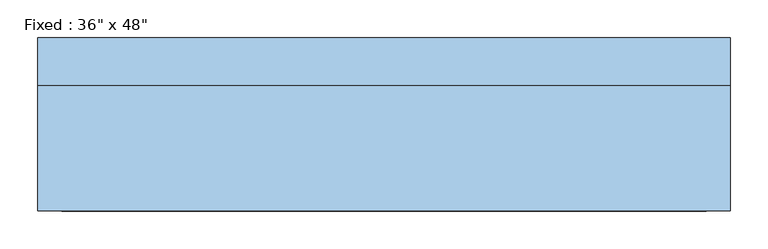
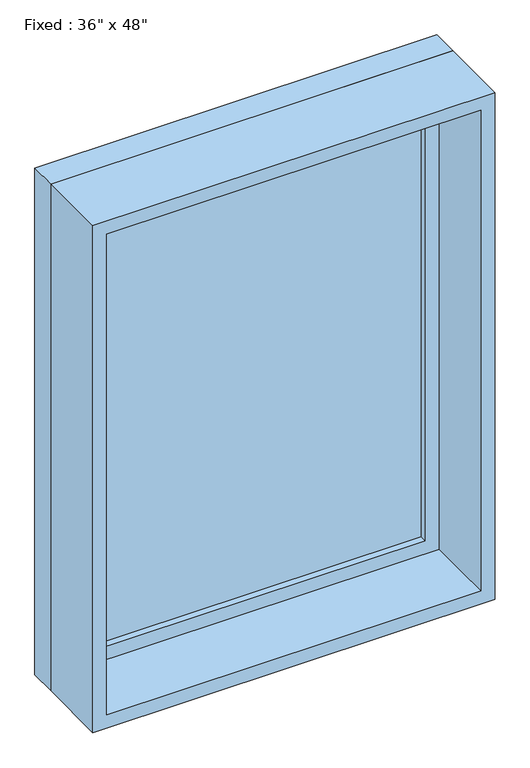
"""IFC4 building model written with IfcOpenShell, lengths in millimetres: window geometry."""

from ifc_helpers import new_model, si_unit, frame, origin, place, context, project, spatial, polyline, outline, extrude, source, transform, mapped, element, save


def window_c1f32544(model_context):
    return source(origin(), model_context, "Body", "SweptSolid", [
        extrude(outline(polyline([(355.6, 66.675), (-431.8, 66.675), (-431.8, 79.375), (355.6, 79.375), (355.6, 66.675)])), frame((0.0, 0.0, 977.9), z_axis=(0.0, 0.0, 1.0), x_axis=(1.0, 0.0, 0.0)), (0.0, 0.0, 1.0), 1092.2),
        extrude(outline(polyline([(2114.55, -476.25), (933.45, -476.25), (933.45, 400.05), (2114.55, 400.05), (2114.55, -476.25)]), holes=[polyline([(2070.1, -431.8), (2070.1, 355.6), (977.9, 355.6), (977.9, -431.8), (2070.1, -431.8)])]), frame((0.0, 50.8, 0.0), z_axis=(0.0, 1.0, 0.0), x_axis=(0.0, 0.0, 1.0)), (0.0, 0.0, 1.0), 44.45),
        extrude(outline(polyline([(2133.6, -495.3), (914.4, -495.3), (914.4, 419.1), (2133.6, 419.1), (2133.6, -495.3)]), holes=[polyline([(2101.85, -463.55), (2101.85, 387.35), (946.15, 387.35), (946.15, -463.55), (2101.85, -463.55)])]), frame((0.0, -114.3, 0.0), z_axis=(0.0, 1.0, 0.0), x_axis=(0.0, 0.0, 1.0)), (0.0, 0.0, 1.0), 165.1),
        extrude(outline(polyline([(2133.6, 419.1), (2133.6, -495.3), (914.4, -495.3), (914.4, 419.1), (2133.6, 419.1)]), holes=[polyline([(2114.55, 400.05), (933.45, 400.05), (933.45, -476.25), (2114.55, -476.25), (2114.55, 400.05)])]), frame((0.0, 50.8, 0.0), z_axis=(0.0, 1.0, 0.0), x_axis=(0.0, 0.0, 1.0)), (0.0, 0.0, 1.0), 63.5),
    ])


if __name__ == "__main__":
    model = new_model("IFC4")
    model_context = context("Model", 3, world=origin())
    ifc_project = project(units=[si_unit("LENGTHUNIT", "METRE", prefix="MILLI")], contexts=[model_context])
    site = spatial("IfcSite", under=ifc_project)
    building = spatial("IfcBuilding", under=site)
    placement = place(None, origin())
    window_shape = window_c1f32544(model_context)
    element("IfcWindow", 1, ObjectType="Fixed : 36\" x 48\"", at=placement, inside=building, context=model_context, shape_type="MappedRepresentation", body=[
        mapped(window_shape, transform((0.0, 0.0, 0.0), x_axis=(1.0, 0.0, 0.0), y_axis=(0.0, 1.0, 0.0), z_axis=(0.0, 0.0, 1.0))),
    ])
    save(model, "model.ifc")

# Revit data of these elements
# Type "Fixed : 36\" x 48\""
#   Type Mark = "1"
#   Construction Type Id = "GSP4R"
#   Assembly Code = "B2020100"
#   Analytic Construction = "1/8 in Pilkington single glazing"
#   Visual Light Transmittance = 0.9
#   Solar Heat Gain Coefficient = 0.78
#   Heat Transfer Coefficient (U) = 0.6496 BTU/(h·ft²·°F)
#   Height = 4' - 0"
#   Default Sill Height = 3' - 0"
#   Width = 3' - 0"
#   Window Inset = 0' - 0 3/4"
#   Define Thermal Properties by = 1
#   Define Thermal Properties by = 1
#   Glass Pane Material = Glass
#   Sash Material = Sash
#   Wall Closure = (empty or 0)
# Element 1 (IfcWindow, "Fixed : 36\" x 48\"")
#   Materials on its faces: "Sash", "Glass"
# Materials
#   "Glass": class "Glass", colour RGB 0 128 192, transparency 0.75, Description = "Soda Lime Glass", Cost = 0
#   "Sash": class "Wood", colour RGB 224 178 126, transparency 0, Cost = 0
